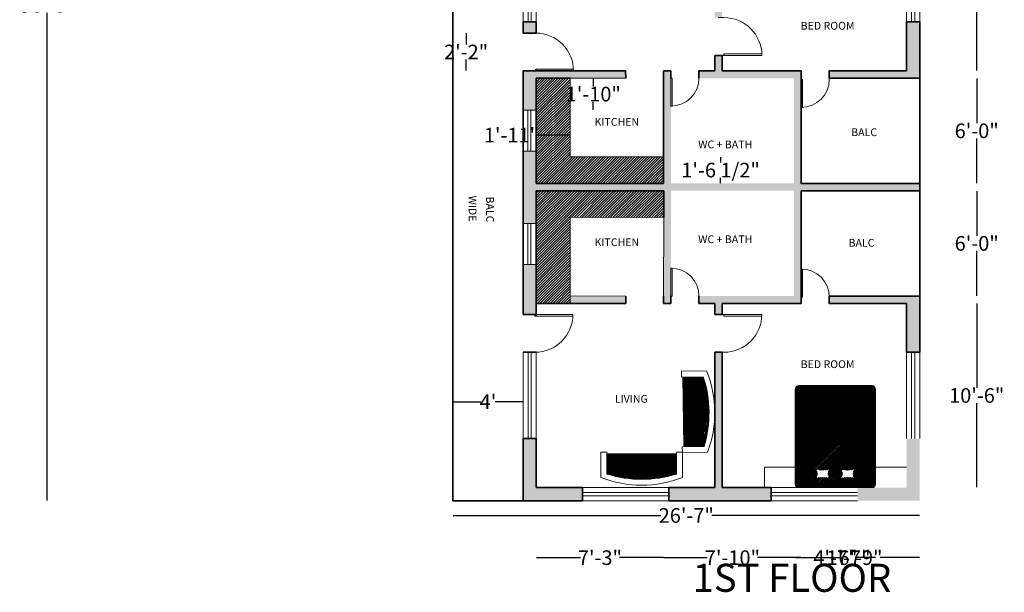
# Model space of a CAD drawing. Units: inches. Extents: x 1198 to 8596, y 144 to 930.
# Tile 1 of 5: x 1270 to 1943, y 144 to 536. Entities that reach past the tile are written whole.
import ezdxf

# ---------------------------------------------------------------- set-up
doc = ezdxf.new("R2010")
doc.units = ezdxf.units.IN
doc.header["$MEASUREMENT"] = 0
doc.layers.get('0').update_dxf_attribs({"color": 50})
for name, color, linetype, lineweight in [('A-ANNO-DIMS', 7, 'Continuous', 18), ('A-ANNO-TEXT', 7, 'Continuous', 25), ('A-AREA-IDEN', 7, 'Continuous', 18), ('A-DOOR', 120, 'Continuous', 18), ('A-FLOR-FIXT', 8, 'Continuous', 18), ('A-FLOR-FIXT-PATT', 150, 'Continuous', 13), ('A-FURN', 11, 'Continuous', 18), ('A-FURN-PATT', 11, 'Continuous', 13), ('A-WALL-PATT', 150, 'Continuous', 13), ('WALL', 7, 'Continuous', 35), ('WINDOW', 2, 'Continuous', 18)]:
    doc.layers.add(name, color=color, linetype=linetype, lineweight=lineweight)
doc.styles.get("Standard").update_dxf_attribs({"font": 'arial.ttf'})
doc.dimstyles.get("Standard").update_dxf_attribs({"dimtxt": 10, "dimasz": 0.18, "dimexe": 0.18, "dimexo": 0.0625, "dimgap": 0.09, "dimtad": 0, "dimtih": 1, "dimtoh": 1, "dimdec": 0, "dimzin": 0, "dimdsep": 46, "dimlunit": 3, "dimtxsty": 'Standard', "dimcen": 0.09, "dimse1": 1, "dimse2": 1, "dimadec": 0, "dimazin": 0, "dimtfac": 1, "dimtdec": 0, "dimtofl": 0, "dimtmove": 0, "dimatfit": 3, "dimfxl": 1, "dimtolj": 1, "dimtzin": 0, "dimarcsym": 0})

# ---------------------------------------------------------------- blocks, each defined once
blk = doc.blocks.new('*D1')
at = {"layer": 'A-ANNO-DIMS', "color": 0, "lineweight": -2, "transparency": 16777216}
for p, q in [((1566.07, 274.64), (1584.99, 274.64)), ((1613.71, 274.64), (1594.78, 274.64))]:
    blk.add_line(p, q, dxfattribs=at)
at = {"layer": 'A-ANNO-DIMS', "color": 0, "transparency": 16777216}
for points in [[(1566.07, 274.67), (1566.07, 274.61), (1565.89, 274.64)], [(1613.71, 274.67), (1613.71, 274.61), (1613.89, 274.64)]]:
    blk.add_solid(points, dxfattribs=at)
at = {"layer": 'Defpoints', "color": 0, "transparency": 16777216}
for p in [(1565.89, 284.02), (1613.89, 284.02), (1565.89, 274.64)]:
    blk.add_point(p, dxfattribs=at)
at = {"layer": 'A-ANNO-DIMS', "color": 0, "transparency": 16777216, "insert": (1589.89, 274.64), "char_height": 10, "attachment_point": 5}
blk.add_mtext("\\A1;4'", dxfattribs=at)
blk = doc.blocks.new('WD_WIN4')
for p, q in [((-0.5, 0.5), (0.5, 0.5)), ((-0.5, 0.12), (0.5, 0.12)), ((-0.5, -0.12), (0.5, -0.12)), ((-0.5, -0.5), (0.5, -0.5))]:
    blk.add_line(p, q)
blk = doc.blocks.new('*U9')
for p, q in [((0, 0), (0, -6)), ((40, 0), (40, -6))]:
    blk.add_line(p, q)
blk.add_lwpolyline([(0, 0), (0, 40), (1.75, 40), (1.75, 0)], close=True)
blk.add_arc((0, 0), 40, 0, 90)
blk = doc.blocks.new('*U11')
for p, q in [((0, 0), (0, -6)), ((40, 0), (40, -6))]:
    blk.add_line(p, q)
blk.add_lwpolyline([(0, 0), (0, 40), (1.75, 40), (1.75, 0)], close=True)
blk.add_arc((0, 0), 40, 0, 90)
blk = doc.blocks.new('*U10')
for p, q in [((0, 0), (0, -6)), ((-40, 0), (-40, -6))]:
    blk.add_line(p, q)
blk.add_lwpolyline([(0, 0), (0, 40), (-1.75, 40), (-1.75, 0)], close=True)
blk.add_arc((0, 0), 40, 90, 180)
blk = doc.blocks.new('*D17')
at = {"layer": 'A-ANNO-DIMS', "color": 0, "lineweight": -2, "transparency": 16777216}
for p, q in [((1288.75, 884.72), (1288.75, 551.09)), ((1288.75, 207.08), (1288.75, 540.7))]:
    blk.add_line(p, q, dxfattribs=at)
at = {"layer": 'A-ANNO-DIMS', "color": 0, "transparency": 16777216}
for points in [[(1288.72, 884.72), (1288.78, 884.72), (1288.75, 884.9)], [(1288.72, 207.08), (1288.78, 207.08), (1288.75, 206.9)]]:
    blk.add_solid(points, dxfattribs=at)
at = {"layer": 'Defpoints', "color": 0, "transparency": 16777216}
for p in [(1347.89, 884.9), (1288.75, 206.9), (1347.89, 206.9)]:
    blk.add_point(p, dxfattribs=at)
at = {"layer": 'A-ANNO-DIMS', "color": 0, "transparency": 16777216, "insert": (1288.75, 545.9), "char_height": 10, "attachment_point": 5}
blk.add_mtext('\\A1;56\'-6"', dxfattribs=at)
blk = doc.blocks.new('Sofa - Roundback 7 ft.')
for p, q in [((-12.00002, -32.4421), (-12.00003, -6.5971)), ((11.99997, -32.4421), (11.99998, -6.5971)), ((-36.000027, -34), (-36.000027, -11.4696)), ((-35.999844, -13.3819), (35.9998, -13.3819)), ((35.99998, -34), (35.99998, -11.4696)), ((-36.000027, -32.4421), (35.99998, -32.4421))]:
    blk.add_line(p, q)
for points in [[(-36.000027, -34), (-42.000027, -34), (-42.000027, -8)], [(41.99998, -8), (41.99998, -34), (35.99998, -34)]]:
    blk.add_lwpolyline(points)
for centre, radius, start, end in [((0, -114.25), 114.25, 68.43141, 111.5686), ((-0.00001, -127.1968), 121.1968, 72.72033, 107.2797)]:
    blk.add_arc(centre, radius, start, end)
blk = doc.blocks.new('*D19')
at = {"layer": 'A-ANNO-DIMS', "color": 0, "lineweight": -2, "transparency": 16777216}
for p, q in [((1566.07, 196.81), (1708.03, 196.81)), ((1884.71, 196.81), (1742.74, 196.81))]:
    blk.add_line(p, q, dxfattribs=at)
at = {"layer": 'A-ANNO-DIMS', "color": 0, "transparency": 16777216}
for points in [[(1566.07, 196.84), (1566.07, 196.78), (1565.89, 196.81)], [(1884.71, 196.84), (1884.71, 196.78), (1884.89, 196.81)]]:
    blk.add_solid(points, dxfattribs=at)
at = {"layer": 'Defpoints', "color": 0, "transparency": 16777216}
for p in [(1565.89, 206.9), (1884.89, 206.9), (1565.89, 196.81)]:
    blk.add_point(p, dxfattribs=at)
at = {"layer": 'A-ANNO-DIMS', "color": 0, "transparency": 16777216, "insert": (1725.39, 196.81), "char_height": 10, "attachment_point": 5}
blk.add_mtext('\\A1;26\'-7"', dxfattribs=at)
blk = doc.blocks.new('WIN-NARROW-28IN')
for p, q in [((0, 9), (0, 0)), ((28.06, 9), (28.06, 0)), ((0, 5.31), (28.06, 5.31)), ((0, 3.31), (28.06, 3.31))]:
    blk.add_line(p, q)
blk = doc.blocks.new('NIGHTSTAND')
for p, q in [((23.07, 13.96), (0, 13.96)), ((23.07, 0), (23.07, 13.96)), ((1.94, 0), (23.07, 0))]:
    blk.add_line(p, q)
blk = doc.blocks.new('*D44')
at = {"layer": 'A-ANNO-DIMS', "color": 0, "lineweight": -2, "transparency": 16777216}
for p, q in [((1923.84, 626.72), (1923.84, 569.09)), ((1923.84, 501.08), (1923.84, 558.7))]:
    blk.add_line(p, q, dxfattribs=at)
at = {"layer": 'A-ANNO-DIMS', "color": 0, "transparency": 16777216}
for points in [[(1923.81, 626.72), (1923.87, 626.72), (1923.84, 626.9)], [(1923.81, 501.08), (1923.87, 501.08), (1923.84, 500.9)]]:
    blk.add_solid(points, dxfattribs=at)
at = {"layer": 'Defpoints', "color": 0, "transparency": 16777216}
for p in [(1875.89, 626.9), (1923.84, 626.9), (1875.89, 500.9)]:
    blk.add_point(p, dxfattribs=at)
at = {"layer": 'A-ANNO-DIMS', "color": 0, "transparency": 16777216, "insert": (1923.84, 563.9), "char_height": 10, "attachment_point": 5}
blk.add_mtext('\\A1;10\'-6"', dxfattribs=at)
blk = doc.blocks.new('*D45')
at = {"layer": 'A-ANNO-DIMS', "color": 0, "lineweight": -2, "transparency": 16777216}
for p, q in [((1923.84, 495.72), (1923.84, 465.09)), ((1923.84, 424.08), (1923.84, 454.7))]:
    blk.add_line(p, q, dxfattribs=at)
at = {"layer": 'A-ANNO-DIMS', "color": 0, "transparency": 16777216}
for points in [[(1923.81, 495.72), (1923.87, 495.72), (1923.84, 495.9)], [(1923.81, 424.08), (1923.87, 424.08), (1923.84, 423.9)]]:
    blk.add_solid(points, dxfattribs=at)
at = {"layer": 'Defpoints', "color": 0, "transparency": 16777216}
for p in [(1884.89, 495.9), (1923.84, 495.9), (1884.89, 423.9)]:
    blk.add_point(p, dxfattribs=at)
at = {"layer": 'A-ANNO-DIMS', "color": 0, "transparency": 16777216, "insert": (1923.84, 459.9), "char_height": 10, "attachment_point": 5}
blk.add_mtext('\\A1;6\'-0"', dxfattribs=at)
blk = doc.blocks.new('*D46')
at = {"layer": 'A-ANNO-DIMS', "color": 0, "lineweight": -2, "transparency": 16777216}
for p, q in [((1923.84, 418.72), (1923.84, 388.09)), ((1923.84, 347.08), (1923.84, 377.7))]:
    blk.add_line(p, q, dxfattribs=at)
at = {"layer": 'A-ANNO-DIMS', "color": 0, "transparency": 16777216}
for points in [[(1923.81, 418.72), (1923.87, 418.72), (1923.84, 418.9)], [(1923.81, 347.08), (1923.87, 347.08), (1923.84, 346.9)]]:
    blk.add_solid(points, dxfattribs=at)
at = {"layer": 'Defpoints', "color": 0, "transparency": 16777216}
for p in [(1884.89, 418.9), (1923.84, 418.9), (1884.89, 346.9)]:
    blk.add_point(p, dxfattribs=at)
at = {"layer": 'A-ANNO-DIMS', "color": 0, "transparency": 16777216, "insert": (1923.84, 382.9), "char_height": 10, "attachment_point": 5}
blk.add_mtext('\\A1;6\'-0"', dxfattribs=at)
blk = doc.blocks.new('*D47')
at = {"layer": 'A-ANNO-DIMS', "color": 0, "lineweight": -2, "transparency": 16777216}
for p, q in [((1923.84, 341.72), (1923.84, 284.09)), ((1923.84, 216.08), (1923.84, 273.7))]:
    blk.add_line(p, q, dxfattribs=at)
at = {"layer": 'A-ANNO-DIMS', "color": 0, "transparency": 16777216}
for points in [[(1923.81, 341.72), (1923.87, 341.72), (1923.84, 341.9)], [(1923.81, 216.08), (1923.87, 216.08), (1923.84, 215.9)]]:
    blk.add_solid(points, dxfattribs=at)
at = {"layer": 'Defpoints', "color": 0, "transparency": 16777216}
for p in [(1875.89, 341.9), (1923.84, 341.9), (1749.89, 215.9)]:
    blk.add_point(p, dxfattribs=at)
at = {"layer": 'A-ANNO-DIMS', "color": 0, "transparency": 16777216, "insert": (1923.84, 278.9), "char_height": 10, "attachment_point": 5}
blk.add_mtext('\\A1;10\'-6"', dxfattribs=at)
blk = doc.blocks.new('*D48')
at = {"layer": 'A-ANNO-DIMS', "color": 0, "lineweight": -2, "transparency": 16777216}
for p, q in [((1623.07, 167.95), (1653.05, 167.95)), ((1709.71, 167.95), (1679.73, 167.95))]:
    blk.add_line(p, q, dxfattribs=at)
at = {"layer": 'A-ANNO-DIMS', "color": 0, "transparency": 16777216}
for points in [[(1623.07, 167.98), (1623.07, 167.92), (1622.89, 167.95)], [(1709.71, 167.98), (1709.71, 167.92), (1709.89, 167.95)]]:
    blk.add_solid(points, dxfattribs=at)
at = {"layer": 'Defpoints', "color": 0, "transparency": 16777216}
for p in [(1622.89, 341.9), (1709.89, 341.9), (1709.89, 167.95)]:
    blk.add_point(p, dxfattribs=at)
at = {"layer": 'A-ANNO-DIMS', "color": 0, "transparency": 16777216, "insert": (1666.39, 167.95), "char_height": 10, "attachment_point": 5}
blk.add_mtext('\\A1;7\'-3"', dxfattribs=at)
blk = doc.blocks.new('*D49')
at = {"layer": 'A-ANNO-DIMS', "color": 0, "lineweight": -2, "transparency": 16777216}
for p, q in [((1710.07, 167.95), (1739.68, 167.95)), ((1803.75, 167.95), (1774.13, 167.95))]:
    blk.add_line(p, q, dxfattribs=at)
at = {"layer": 'A-ANNO-DIMS', "color": 0, "transparency": 16777216}
for points in [[(1710.07, 167.98), (1710.07, 167.92), (1709.89, 167.95)], [(1803.75, 167.98), (1803.75, 167.92), (1803.93, 167.95)]]:
    blk.add_solid(points, dxfattribs=at)
at = {"layer": 'Defpoints', "color": 0, "transparency": 16777216}
for p in [(1709.89, 341.9), (1803.93, 341.9), (1803.93, 167.95)]:
    blk.add_point(p, dxfattribs=at)
at = {"layer": 'A-ANNO-DIMS', "color": 0, "transparency": 16777216, "insert": (1756.91, 167.95), "char_height": 10, "attachment_point": 5}
blk.add_mtext('\\A1;7\'-10"', dxfattribs=at)
blk = doc.blocks.new('*D50')
at = {"layer": 'A-ANNO-DIMS', "color": 0, "lineweight": -2, "transparency": 16777216}
for p, q in [((1804.07, 167.95), (1830.98, 167.95)), ((1884.71, 167.95), (1857.79, 167.95))]:
    blk.add_line(p, q, dxfattribs=at)
at = {"layer": 'A-ANNO-DIMS', "color": 0, "transparency": 16777216}
for points in [[(1804.07, 167.98), (1804.07, 167.92), (1803.89, 167.95)], [(1884.71, 167.98), (1884.71, 167.92), (1884.89, 167.95)]]:
    blk.add_solid(points, dxfattribs=at)
at = {"layer": 'Defpoints', "color": 0, "transparency": 16777216}
for p in [(1803.89, 346.9), (1884.89, 346.9), (1884.89, 167.95)]:
    blk.add_point(p, dxfattribs=at)
at = {"layer": 'A-ANNO-DIMS', "color": 0, "transparency": 16777216, "insert": (1844.39, 167.95), "char_height": 10, "attachment_point": 5}
blk.add_mtext('\\A1;6\'-9"', dxfattribs=at)
blk = doc.blocks.new('*D51')
at = {"layer": 'A-ANNO-DIMS', "color": 0, "lineweight": -2, "transparency": 16777216}
for p, q in [((1804.07, 167.95), (1822.93, 167.95)), ((1823.11, 167.95), (1823.29, 167.95))]:
    blk.add_line(p, q, dxfattribs=at)
at = {"layer": 'A-ANNO-DIMS', "color": 0, "transparency": 16777216}
for points in [[(1804.07, 167.98), (1804.07, 167.92), (1803.89, 167.95)], [(1822.93, 167.98), (1822.93, 167.92), (1823.11, 167.95)]]:
    blk.add_solid(points, dxfattribs=at)
at = {"layer": 'Defpoints', "color": 0, "transparency": 16777216}
for p in [(1803.89, 495.9), (1823.11, 495.9), (1823.11, 167.95)]:
    blk.add_point(p, dxfattribs=at)
at = {"layer": 'A-ANNO-DIMS', "color": 0, "transparency": 16777216, "insert": (1836.2, 167.95), "char_height": 10, "attachment_point": 5}
blk.add_mtext('\\A1;1\'-7"', dxfattribs=at)
blk = doc.blocks.new('*D52')
at = {"layer": 'A-ANNO-DIMS', "color": 0, "lineweight": -2, "transparency": 16777216}
for p, q in [((1574.94, 526.59), (1574.94, 518.95)), ((1574.94, 501.08), (1574.94, 508.72))]:
    blk.add_line(p, q, dxfattribs=at)
at = {"layer": 'A-ANNO-DIMS', "color": 0, "transparency": 16777216}
for points in [[(1574.91, 526.59), (1574.97, 526.59), (1574.94, 526.77)], [(1574.91, 501.08), (1574.97, 501.08), (1574.94, 500.9)]]:
    blk.add_solid(points, dxfattribs=at)
at = {"layer": 'Defpoints', "color": 0, "transparency": 16777216}
for p in [(1574.94, 526.77), (1613.89, 526.77), (1613.89, 500.9)]:
    blk.add_point(p, dxfattribs=at)
at = {"layer": 'A-ANNO-DIMS', "color": 0, "transparency": 16777216, "insert": (1574.94, 513.84), "char_height": 10, "attachment_point": 5}
blk.add_mtext('\\A1;2\'-2"', dxfattribs=at)
blk = doc.blocks.new('*D53')
at = {"layer": 'A-ANNO-DIMS', "color": 0, "lineweight": -2, "transparency": 16777216}
for p, q in [((1800.03, 167.95), (1813.72, 167.95)), ((1854.57, 167.95), (1840.88, 167.95))]:
    blk.add_line(p, q, dxfattribs=at)
at = {"layer": 'A-ANNO-DIMS', "color": 0, "transparency": 16777216}
for points in [[(1800.03, 167.98), (1800.03, 167.92), (1799.85, 167.95)], [(1854.57, 167.98), (1854.57, 167.92), (1854.75, 167.95)]]:
    blk.add_solid(points, dxfattribs=at)
at = {"layer": 'Defpoints', "color": 0, "transparency": 16777216}
for p in [(1799.85, 559.62), (1854.75, 559.62), (1854.75, 167.95)]:
    blk.add_point(p, dxfattribs=at)
at = {"layer": 'A-ANNO-DIMS', "color": 0, "transparency": 16777216, "insert": (1827.3, 167.95), "char_height": 10, "attachment_point": 5}
blk.add_mtext('\\A1;4\'-7"', dxfattribs=at)
blk = doc.blocks.new('*D62')
at = {"layer": 'A-ANNO-DIMS', "color": 0, "lineweight": -2, "transparency": 16777216}
for p, q in [((1622.89, 456.95), (1622.71, 456.95)), ((1645.75, 456.95), (1623.07, 456.95))]:
    blk.add_line(p, q, dxfattribs=at)
at = {"layer": 'A-ANNO-DIMS', "color": 0, "transparency": 16777216}
for points in [[(1623.07, 456.98), (1623.07, 456.92), (1622.89, 456.95)], [(1645.75, 456.98), (1645.75, 456.92), (1645.93, 456.95)]]:
    blk.add_solid(points, dxfattribs=at)
at = {"layer": 'Defpoints', "color": 0, "transparency": 16777216}
for p in [(1622.89, 495.9), (1645.93, 495.9), (1622.89, 456.95)]:
    blk.add_point(p, dxfattribs=at)
at = {"layer": 'A-ANNO-DIMS', "color": 0, "transparency": 16777216, "insert": (1605.91, 456.95), "char_height": 10, "attachment_point": 5}
blk.add_mtext('\\A1;1\'-11"', dxfattribs=at)
blk = doc.blocks.new('*D63')
at = {"layer": 'A-ANNO-DIMS', "color": 0, "lineweight": -2, "transparency": 16777216}
for p, q in [((1748.84, 441.97), (1748.84, 438.28)), ((1748.84, 424.08), (1748.84, 427.76))]:
    blk.add_line(p, q, dxfattribs=at)
at = {"layer": 'A-ANNO-DIMS', "color": 0, "transparency": 16777216}
for points in [[(1748.81, 441.97), (1748.87, 441.97), (1748.84, 442.15)], [(1748.81, 424.08), (1748.87, 424.08), (1748.84, 423.9)]]:
    blk.add_solid(points, dxfattribs=at)
at = {"layer": 'Defpoints', "color": 0, "transparency": 16777216}
for p in [(1709.89, 442.15), (1709.89, 423.9), (1748.84, 423.9)]:
    blk.add_point(p, dxfattribs=at)
at = {"layer": 'A-ANNO-DIMS', "color": 0, "transparency": 16777216, "insert": (1748.84, 433.02), "char_height": 10, "attachment_point": 5}
blk.add_mtext('\\A1;1\'-6 1/2"', dxfattribs=at)
blk = doc.blocks.new('*D67')
at = {"layer": 'A-ANNO-DIMS', "color": 0, "lineweight": -2, "transparency": 16777216}
for p, q in [((1661.84, 495.72), (1661.84, 490.21)), ((1661.84, 474.31), (1661.84, 479.82))]:
    blk.add_line(p, q, dxfattribs=at)
at = {"layer": 'A-ANNO-DIMS', "color": 0, "transparency": 16777216}
for points in [[(1661.81, 495.72), (1661.87, 495.72), (1661.84, 495.9)], [(1661.81, 474.31), (1661.87, 474.31), (1661.84, 474.13)]]:
    blk.add_solid(points, dxfattribs=at)
at = {"layer": 'Defpoints', "color": 0, "transparency": 16777216}
for p in [(1622.89, 495.9), (1622.89, 474.13), (1661.84, 474.13)]:
    blk.add_point(p, dxfattribs=at)
at = {"layer": 'A-ANNO-DIMS', "color": 0, "transparency": 16777216, "insert": (1661.84, 485.01), "char_height": 10, "attachment_point": 5}
blk.add_mtext('\\A1;1\'-10"', dxfattribs=at)

msp = doc.modelspace()

# ---------------------------------------------------------------- hatches: boundary and pattern name
at = {"layer": 'A-FLOR-FIXT-PATT'}
h = msp.add_hatch(dxfattribs=at)
h.set_pattern_fill('ANSI31', color=256, scale=10)
h.paths.add_polyline_path([(1646.14, 400.75), (1710.09, 400.51), (1710.09, 418.9), (1622.89, 418.9), (1622.89, 341.9), (1645.93, 341.9), (1645.93, 347.01)])
h.paths.add_polyline_path([(1709.89, 442.15), (1645.93, 442.15), (1645.93, 495.9), (1622.89, 495.9), (1622.89, 423.9), (1709.89, 423.9)])
at = {"layer": 'A-FURN-PATT'}
h = msp.add_hatch(dxfattribs=at)
h.set_pattern_fill('LINE', color=256, scale=5, angle=90.6803)
h.set_pattern_definition([(90.6803, (2441.98376, -1260.8571), (-0.62495594, -0.00742075), [])])
h.paths.add_polyline_path([(1723.51, 259.75), (1723.69, 243.86), (1736.31, 244.01), (1736.12, 259.9)])
h.paths.add_polyline_path([(1723.32, 275.63), (1723.51, 259.75), (1736.12, 259.9), (1735.93, 275.78)])
h.paths.add_polyline_path([(1723.13, 291.52), (1723.32, 275.63), (1735.93, 275.78), (1735.75, 291.67)])
h.paths.add_polyline_path([(1737.01, 291.69), (1735.75, 291.67), (1735.93, 275.78), (1740.43, 275.84, 0.050647)])
h.paths.add_polyline_path([(1735.93, 275.78), (1736.12, 259.9), (1740.61, 259.95, 0.049628), (1740.43, 275.84)])
h.paths.add_polyline_path([(1736.12, 259.9), (1736.31, 244.01), (1737.58, 244.03, 0.050647), (1740.61, 259.95)])
h = msp.add_hatch(dxfattribs=at)
h.set_pattern_fill('PLASTI', color=256, scale=6.190048)
h.set_pattern_definition([(0, (526.78, -195.5534), (0, 1.547512), []), (0, (526.78, -195.36), (0, 1.547512), []), (0, (526.78, -195.1665), (0, 1.547512), []), (0, (526.78, -194.5862), (0, 1.547512), [])])
h.paths.add_polyline_path([(1846.77, 215.84), (1852.27, 215.84, 0.414214), (1854.75, 218.31), (1854.75, 283.17, 0.414214), (1852.27, 285.65), (1846.77, 285.65)])
h.paths.add_polyline_path([(1799.85, 218.31, 0.414214), (1802.33, 215.84), (1807.83, 215.84), (1807.83, 285.65), (1802.33, 285.65, 0.414214), (1799.85, 283.17)])
h = msp.add_hatch(dxfattribs=at)
h.set_pattern_fill('ANSI38', color=256, scale=6.190048)
h.set_pattern_definition([(45, (526.78, -195.5534), (-0.5471281, 0.5471281), []), (135, (526.78, -195.5534), (-1.6413843, 0.5471281), [1.93439, -1.160634])])
h.paths.add_polyline_path([(1807.83, 215.84), (1846.77, 215.84), (1846.77, 285.65), (1807.83, 285.65)])
h.paths.add_polyline_path([(1823.26, 228.35, 0.358285), (1823.26, 222.35, 0.116256), (1813.93, 222.35, 0.358285), (1813.93, 228.35, 0.116256)], flags=16)
h.paths.add_polyline_path([(1831.01, 228.35, 0.116256), (1840.34, 228.35, 0.358285), (1840.34, 222.35, 0.116256), (1831.01, 222.35, 0.358285)], flags=16)
h = msp.add_hatch(dxfattribs=at)
h.set_pattern_fill('LINE', color=256, scale=5)
h.set_pattern_definition([(0, (157.9337, -461.3583), (0, 0.625), [])])
h.paths.add_polyline_path([(1686.96, 239.01), (1671.07, 239.01), (1671.07, 226.4), (1686.96, 226.4)])
h.paths.add_polyline_path([(1702.85, 239.01), (1686.96, 239.01), (1686.96, 226.4), (1702.85, 226.4)])
h.paths.add_polyline_path([(1718.74, 239.01), (1702.85, 239.01), (1702.85, 226.4), (1718.74, 226.4)])
h.paths.add_polyline_path([(1718.74, 225.13), (1718.74, 226.4), (1702.85, 226.4), (1702.85, 221.9, 0.050647)])
h.paths.add_polyline_path([(1702.85, 226.4), (1686.96, 226.4), (1686.96, 221.9, 0.049628), (1702.85, 221.9)])
h.paths.add_polyline_path([(1686.96, 226.4), (1671.07, 226.4), (1671.07, 225.13, 0.050647), (1686.96, 221.9)])
at = {"layer": 'A-WALL-PATT'}
h = msp.add_hatch(color=256, dxfattribs=at)
h.dxf.hatch_style = 1
h.paths.add_polyline_path([(1884.89, 495.9), (1884.89, 534.37), (1875.89, 534.37), (1875.89, 500.9), (1823.11, 500.9), (1823.11, 495.9)])
h.paths.add_polyline_path([(1875.89, 593.42), (1884.89, 593.42), (1884.89, 685.87), (1875.89, 685.87), (1875.89, 631.9), (1749.89, 631.9), (1749.89, 766.08), (1744.89, 766.08), (1744.89, 631.97), (1618.79, 631.97), (1613.89, 631.97), (1613.89, 593.42), (1622.89, 593.42), (1622.89, 626.9), (1744.89, 626.9), (1744.89, 537.33), (1749.89, 537.33), (1749.89, 626.9), (1875.89, 626.9)])
h.paths.add_polyline_path([(1884.89, 206.9), (1884.89, 249.37), (1875.89, 249.37), (1875.89, 215.9), (1842.41, 215.9), (1842.41, 206.9)])
h.paths.add_polyline_path([(1783.36, 206.9), (1783.36, 215.9), (1749.89, 215.9), (1749.89, 308.42), (1744.89, 308.42), (1744.89, 215.9), (1713.41, 215.9), (1713.41, 206.9)])
h.paths.add_polyline_path([(1654.36, 206.9), (1654.36, 215.9), (1622.89, 215.9), (1622.89, 249.37), (1613.89, 249.37), (1613.89, 206.9)])
h.paths.add_polyline_path([(1613.89, 334.34), (1622.89, 334.34), (1622.89, 341.9), (1622.89, 368.41), (1613.89, 368.41)])
h.paths.add_polyline_path([(1613.89, 396.47), (1622.89, 396.47), (1622.89, 418.9), (1710.09, 418.9), (1710.09, 400.51), (1709.89, 346.77), (1709.89, 341.9), (1714.89, 341.9), (1714.89, 346.9), (1714.88, 366), (1714.89, 418.9), (1798.89, 418.9), (1798.89, 346.9), (1734.06, 346.9), (1734.07, 343.96), (1734.06, 341.9), (1744.89, 341.9), (1744.89, 334.34), (1749.89, 334.34), (1749.89, 341.9), (1803.93, 341.9), (1803.93, 346.9), (1803.89, 346.9), (1803.89, 418.9), (1884.89, 418.9), (1884.89, 423.9), (1803.89, 423.9), (1803.89, 495.9), (1803.93, 500.9), (1749.89, 500.9), (1749.89, 511.41), (1747.24, 511.41), (1744.89, 511.41), (1744.89, 500.9), (1734.06, 500.9), (1734.06, 495.9), (1798.89, 495.9), (1798.89, 423.9), (1714.89, 423.9), (1714.89, 495.9), (1714.89, 500.9), (1709.89, 500.9), (1709.89, 496.89), (1709.89, 495.9), (1709.89, 423.9), (1622.89, 423.9), (1622.89, 446.07), (1613.89, 446.07)])
h.paths.add_polyline_path([(1613.89, 474.13), (1622.89, 474.13), (1622.89, 495.9), (1645.93, 495.9), (1683.97, 495.9), (1683.89, 500.9), (1648.32, 500.9), (1648.32, 500.88), (1622.41, 500.86), (1618.52, 500.86), (1613.89, 500.9)])
h.paths.add_polyline_path([(1613.89, 526.77), (1613.89, 534.37), (1622.89, 534.37), (1622.89, 526.77, -0.395914), (1648.3, 502.01), (1648.32, 502.01), (1648.32, 500.88), (1622.41, 500.86), (1622.41, 502), (1648.3, 502.01, 0.395914), (1622.89, 526.77)])
h.paths.add_polyline_path([(1875.89, 744.92), (1884.89, 744.92), (1884.89, 803.9), (1823.06, 803.9), (1823.06, 798.9), (1875.89, 798.9)])
h.paths.add_polyline_path([(1798.89, 803.9), (1734.06, 803.9), (1734.06, 802.45), (1734.06, 798.9), (1744.89, 798.9), (1744.89, 792), (1749.89, 792), (1749.89, 798.9), (1803.89, 798.9), (1803.89, 803.9), (1803.89, 884.9), (1774.16, 884.9), (1774.16, 875.9), (1798.89, 875.9)])
h.paths.add_polyline_path([(1746.09, 875.9), (1746.09, 884.9), (1693.91, 884.9), (1693.91, 875.9), (1709.89, 875.9), (1709.89, 803.9), (1709.89, 798.9), (1714.89, 798.9), (1714.89, 803.9), (1714.89, 875.9)])
h.paths.add_polyline_path([(1618.89, 798.9), (1683.96, 798.9), (1683.96, 803.9), (1618.89, 803.9), (1618.89, 875.9), (1634.86, 875.9), (1634.86, 884.9), (1597.91, 884.9), (1597.91, 875.9), (1613.89, 875.9), (1613.89, 803.9), (1548.75, 803.9), (1548.75, 798.9), (1613.89, 798.9), (1613.89, 657.88), (1618.8, 657.88)])
h.paths.add_polyline_path([(1522.89, 875.9), (1538.86, 875.9), (1538.86, 884.9), (1483.76, 884.9), (1483.76, 875.9), (1517.89, 875.9), (1517.89, 803.9), (1517.89, 802.46), (1517.89, 798.9), (1522.89, 798.9), (1522.89, 803.9)], flags=17)
h.paths.add_polyline_path([(1428.89, 884.9), (1428.89, 803.9), (1428.89, 798.9), (1482.89, 798.9), (1482.89, 678.9), (1356.89, 678.9), (1356.89, 709.37), (1347.89, 709.37), (1347.89, 577.9), (1508.89, 577.9), (1508.89, 586.9), (1356.89, 586.9), (1356.89, 673.9), (1565.89, 673.9), (1565.89, 678.9), (1487.89, 678.9), (1487.89, 798.9), (1498.72, 798.9), (1498.72, 803.9), (1433.89, 803.9), (1433.89, 875.9), (1455.69, 875.9), (1455.69, 884.9)])
h.paths.add_polyline_path([(1356.89, 798.9), (1409.72, 798.9), (1409.72, 803.9), (1347.89, 803.9), (1347.89, 768.42), (1356.89, 768.42)], flags=17)
h.paths.add_polyline_path([(1884.89, 346.9), (1823.09, 346.9, -0.008805), (1823.1, 346.22), (1823.11, 343.35), (1823.09, 341.9), (1875.89, 341.9), (1875.89, 308.42), (1884.89, 308.42)])
h = msp.add_hatch(color=256, dxfattribs=at)
h.dxf.hatch_style = 1
h.paths.add_polyline_path([(1683.97, 346.87), (1645.93, 347.01), (1645.93, 341.9), (1683.97, 341.9)])

# ---------------------------------------------------------------- linework, layer by layer
at = {"layer": 'A-FLOR-FIXT'}
msp.add_line((1645.93, 347.01), (1645.93, 341.9), dxfattribs=at)
for points in [[(1709.89, 495.9), (1709.89, 495.9), (1709.89, 442.15), (1645.93, 442.15), (1645.93, 495.9), (1683.97, 495.9)], [(1709.89, 346.77), (1710.09, 400.51), (1646.14, 400.75), (1645.93, 347.01), (1683.97, 346.87)]]:
    msp.add_lwpolyline(points, dxfattribs=at)
at = {"layer": 'A-FURN'}
for p, q in [((1807.83, 215.84), (1807.83, 285.65)), ((1846.77, 215.84), (1846.77, 285.65)), ((1854.75, 229.85), (1875.89, 229.85))]:
    msp.add_line(p, q, dxfattribs=at)
msp.add_lwpolyline([(1802.33, 215.84), (1852.27, 215.84, 0.414214), (1854.75, 218.31), (1854.75, 283.17, 0.414214), (1852.27, 285.65), (1802.33, 285.65, 0.414214), (1799.85, 283.17), (1799.85, 218.31, 0.414214)], format="xyb", close=True, dxfattribs=at)
at = {"layer": 'WALL'}
for p, q in [((1565.89, 577.9), (1565.89, 206.9)), ((1613.89, 534.37), (1613.89, 526.77)), ((1622.89, 534.37), (1613.89, 534.37)), ((1622.89, 526.77), (1622.89, 534.37)), ((1875.89, 500.9), (1875.89, 534.37)), ((1875.89, 534.37), (1884.89, 534.37)), ((1884.89, 308.42), (1884.89, 534.37)), ((1622.89, 526.77), (1613.89, 526.77)), ((1744.89, 500.9), (1744.89, 511.41)), ((1749.89, 511.41), (1744.89, 511.41)), ((1749.89, 500.9), (1749.89, 511.41)), ((1622.89, 500.9), (1613.89, 500.9)), ((1613.89, 500.9), (1613.89, 334.34)), ((1622.89, 500.9), (1622.89, 502)), ((1622.89, 500.9), (1683.89, 500.9)), ((1683.97, 495.9), (1683.89, 500.9)), ((1709.89, 496.89), (1709.89, 500.9)), ((1709.89, 500.9), (1714.89, 500.9)), ((1714.89, 495.97), (1714.89, 500.9)), ((1734.06, 495.9), (1734.06, 500.9)), ((1734.06, 500.9), (1744.89, 500.9)), ((1749.89, 500.9), (1803.93, 500.9)), ((1803.93, 495.9), (1803.93, 500.9)), ((1823.11, 495.9), (1823.11, 500.9)), ((1823.11, 500.9), (1875.89, 500.9)), ((1622.89, 423.9), (1622.89, 495.9)), ((1622.89, 495.9), (1645.93, 495.9)), ((1709.89, 496.89), (1709.89, 495.9)), ((1709.89, 495.9), (1709.89, 423.9)), ((1803.89, 495.9), (1803.93, 495.9)), ((1803.89, 423.9), (1803.89, 495.9)), ((1823.11, 495.9), (1884.89, 495.9)), ((1709.89, 423.9), (1622.89, 423.9)), ((1803.89, 423.9), (1884.89, 423.9)), ((1710.09, 418.9), (1622.89, 418.9)), ((1622.89, 418.9), (1622.89, 341.9)), ((1710.09, 400.51), (1710.09, 418.9)), ((1803.89, 346.9), (1803.89, 418.9)), ((1803.89, 418.9), (1884.89, 418.9)), ((1683.97, 346.9), (1683.97, 341.9)), ((1709.89, 346.9), (1709.89, 341.9)), ((1714.89, 346.9), (1714.89, 341.9)), ((1734.06, 346.9), (1734.06, 341.9)), ((1803.89, 346.9), (1804.77, 346.9)), ((1803.93, 346.9), (1803.93, 341.9)), ((1823.09, 346.9), (1823.09, 341.9)), ((1823.09, 346.9), (1884.89, 346.9)), ((1622.89, 341.9), (1683.97, 341.9)), ((1622.89, 333.21), (1622.89, 341.9)), ((1709.89, 341.9), (1714.89, 341.9)), ((1734.06, 341.9), (1744.89, 341.9)), ((1744.89, 334.34), (1744.89, 341.9)), ((1749.89, 341.9), (1803.93, 341.9)), ((1749.89, 334.34), (1749.89, 341.9)), ((1823.09, 341.9), (1875.89, 341.9)), ((1875.89, 308.42), (1875.89, 341.9)), ((1622.89, 334.34), (1613.89, 334.34)), ((1749.89, 334.34), (1744.89, 334.34)), ((1622.89, 308.42), (1613.89, 308.42)), ((1622.89, 308.42), (1622.89, 308.44)), ((1744.89, 215.9), (1744.89, 308.42)), ((1749.89, 308.42), (1744.89, 308.42)), ((1749.89, 215.9), (1749.89, 308.42)), ((1875.89, 308.42), (1884.89, 308.42)), ((1613.89, 249.37), (1613.89, 206.9)), ((1622.89, 249.37), (1613.89, 249.37)), ((1622.89, 215.9), (1622.89, 249.37)), ((1622.89, 215.9), (1654.36, 215.9)), ((1654.36, 215.9), (1654.36, 206.9)), ((1713.41, 215.9), (1744.89, 215.9)), ((1713.41, 215.9), (1713.41, 206.9)), ((1749.89, 215.9), (1783.36, 215.9)), ((1783.36, 215.9), (1783.36, 206.9)), ((1565.89, 206.9), (1654.36, 206.9)), ((1713.41, 206.9), (1783.36, 206.9))]:
    msp.add_line(p, q, dxfattribs=at)

# ---------------------------------------------------------------- block references
at = {"layer": 'A-DOOR'}
for name, p, xscale, yscale, zscale, rotation in [('*U10', (1751.13, 511.41), 0.6478828703427376, 0.6478828703427376, 0.6478828703427376, 270.0341043339827), ('*U10', (1622.41, 500.86), 0.6478828703427376, 0.6478828703427376, 0.6478828703427376, 270.0341043339827), ('*U11', (1714.89, 495.97), -0.4792807635590344, 0.4792807635590344, 0.4792807635590344, 179.9658956660211), ('*U11', (1803.93, 495.09), -0.4792807635590344, 0.4792807635590344, 0.4792807635590344, 179.9658956660211), ('*U11', (1714.89, 346.82), 0.4792807635590344, 0.4792807635590344, 0.4792807635590344, 0.0341043339915428), ('*U11', (1803.93, 346.21), 0.4792807635590344, 0.4792807635590344, 0.4792807635590344, 0.0341043339915428), ('*U9', (1621.98, 334.34), 0.6478828703427376, 0.6478828703427376, 0.6478828703427376, 270), ('*U9', (1751.09, 334.34), 0.6478828703427376, 0.6478828703427376, 0.6478828703427376, 270)]:
    msp.add_blockref(name, p, dxfattribs=dict(at, xscale=xscale, yscale=yscale, zscale=zscale, rotation=rotation))
at = {"layer": 'A-FURN', "xscale": 0.6619781710857556, "yscale": 0.6619781710857556, "zscale": 0.6619781710857556}
for p, rotation in [((1744.89, 267.95), 270.6803002411188), ((1694.91, 217.54), 179.9999999999996)]:
    msp.add_blockref('Sofa - Roundback 7 ft.', p, dxfattribs=dict(at, rotation=rotation))
at = {"layer": 'A-FURN', "rotation": 180}
msp.add_blockref('NIGHTSTAND', (1801.79, 229.85), dxfattribs=at)
at = {"layer": 'WINDOW', "xscale": 59.05511811023622, "zscale": 59.05511811023622}
for p, yscale, rotation in [((1618.39, 563.9), 8.999999999999773, 90.00000000000351), ((1880.39, 563.9), 8.999999999988859, 270.0000000000092), ((1618.39, 278.9), 8.999999999982945, 90.00000000000043), ((1880.39, 278.9), 8.999999999998863, 270.0000000000002), ((1683.89, 211.4), 8.999999999972289, 9.0446e-12), ((1812.89, 211.4), 9.000000000001336, 180.0000000000002)]:
    msp.add_blockref('WD_WIN4', p, dxfattribs=dict(at, yscale=yscale, rotation=rotation))
at = {"layer": 'WINDOW', "rotation": 270.0000000000001}
for p in [(1613.89, 474.13), (1613.89, 396.47)]:
    msp.add_blockref('WIN-NARROW-28IN', p, dxfattribs=at)

# ---------------------------------------------------------------- texts
at = {"layer": 'A-ANNO-TEXT'}
msp.add_text('1ST FLOOR', height=19.187, dxfattribs=at).set_placement((1729.68, 144.57))
at = {"layer": 'A-AREA-IDEN'}
for s, p in [(' BED ROOM', (1801.94, 529.13)), (' KITCHEN', (1661.06, 463.35)), ('BALC', (1838.07, 456.29)), ('WC + BATH', (1733.51, 447.94)), (' KITCHEN', (1661.06, 381.02)), ('WC + BATH', (1733.51, 383.09)), ('BALC', (1836.29, 380.66)), (' BED ROOM', (1801.94, 297.64)), (' LIVING', (1674.94, 273.88))]:
    msp.add_text(s, height=5.299, dxfattribs=at).set_placement(p)
for s, p in [(' WIDE', (1576.71, 417.23)), ('BALC', (1588.61, 414.93))]:
    msp.add_text(s, height=5.299, rotation=270, dxfattribs=at).set_placement(p)

# ---------------------------------------------------------------- dimensions: what is measured, and where the dimension line sits
at = {"layer": 'A-ANNO-DIMS'}
for base, p1, p2, angle, override, picture, middle in [((1288.75, 206.9), (1347.89, 884.9), (1347.89, 206.9), 90, {"dimclrd": 0, "dimclre": 0, "dimclrt": 0}, '*D17', (1288.75, 545.9)), ((1923.84, 626.9), (1875.89, 500.9), (1875.89, 626.9), 90, {"dimdec": 1, "dimlfac": 1, "dimrnd": 0, "dimzin": 1, "dimdsep": 46, "dimlunit": 4, "dimfrac": 2}, '*D44', (1923.84, 563.9)), ((1574.94, 526.77), (1613.89, 500.9), (1613.89, 526.77), 90, {"dimdec": 1, "dimlfac": 1, "dimrnd": 0, "dimzin": 1, "dimdsep": 46, "dimlunit": 4, "dimfrac": 2}, '*D52', (1574.94, 513.84)), ((1622.89, 456.95), (1645.93, 495.9), (1622.89, 495.9), 180, {"dimdec": 1, "dimlfac": 1, "dimrnd": 0, "dimzin": 1, "dimdsep": 46, "dimlunit": 4, "dimfrac": 2}, '*D62', (1605.91, 456.95)), ((1661.84, 474.13), (1622.89, 495.9), (1622.89, 474.13), 270, {"dimdec": 1, "dimlfac": 1, "dimrnd": 0, "dimzin": 1, "dimdsep": 46, "dimlunit": 4, "dimfrac": 2}, '*D67', (1661.84, 485.01)), ((1923.84, 495.9), (1884.89, 423.9), (1884.89, 495.9), 90, {"dimdec": 1, "dimlfac": 1, "dimrnd": 0, "dimzin": 1, "dimdsep": 46, "dimlunit": 4, "dimfrac": 2}, '*D45', (1923.84, 459.9)), ((1748.8363, 423.8966), (1709.8863, 442.1522), (1709.8863, 423.8966), 270, {"dimdec": 1, "dimlfac": 1, "dimrnd": 0, "dimzin": 1, "dimdsep": 46, "dimlunit": 4, "dimfrac": 2}, '*D63', (1748.8363, 433.0244)), ((1923.84, 418.9), (1884.89, 346.9), (1884.89, 418.9), 90, {"dimdec": 1, "dimlfac": 1, "dimrnd": 0, "dimzin": 1, "dimdsep": 46, "dimlunit": 4, "dimfrac": 2}, '*D46', (1923.84, 382.9)), ((1923.84, 341.9), (1749.89, 215.9), (1875.89, 341.9), 90, {"dimdec": 1, "dimlfac": 1, "dimrnd": 0, "dimzin": 1, "dimdsep": 46, "dimlunit": 4, "dimfrac": 2}, '*D47', (1923.84, 278.9))]:
    dim = msp.add_linear_dim(base=base, p1=p1, p2=p2, angle=angle, dimstyle='Standard', override=override, dxfattribs=at)
    dim.commit()
    dim.dimension.update_dxf_attribs({"geometry": picture, "text_midpoint": middle})
for base, p1, p2, override, picture, middle in [((1854.75, 167.95), (1799.85, 559.62), (1854.75, 559.62), {"dimdec": 1, "dimlfac": 1, "dimrnd": 0, "dimzin": 1, "dimdsep": 46, "dimlunit": 4, "dimfrac": 2}, '*D53', (1827.3, 167.95)), ((1823.11, 167.95), (1803.89, 495.9), (1823.11, 495.9), {"dimdec": 1, "dimlfac": 1, "dimrnd": 0, "dimzin": 1, "dimdsep": 46, "dimlunit": 4, "dimfrac": 2}, '*D51', (1836.2, 167.95)), ((1884.89, 167.95), (1803.89, 346.9), (1884.89, 346.9), {"dimdec": 1, "dimlfac": 1, "dimrnd": 0, "dimzin": 1, "dimdsep": 46, "dimlunit": 4, "dimfrac": 2}, '*D50', (1844.39, 167.95)), ((1709.89, 167.95), (1622.89, 341.9), (1709.89, 341.9), {"dimdec": 1, "dimlfac": 1, "dimrnd": 0, "dimzin": 1, "dimdsep": 46, "dimlunit": 4, "dimfrac": 2}, '*D48', (1666.39, 167.95)), ((1803.93, 167.95), (1709.89, 341.9), (1803.93, 341.9), {"dimdec": 1, "dimlfac": 1, "dimrnd": 0, "dimzin": 1, "dimdsep": 46, "dimlunit": 4, "dimfrac": 2}, '*D49', (1756.91, 167.95)), ((1565.89, 274.64), (1613.89, 284.02), (1565.89, 284.02), {"dimclrd": 0, "dimclre": 0, "dimclrt": 0}, '*D1', (1589.89, 274.64)), ((1565.89, 196.81), (1884.89, 206.9), (1565.89, 206.9), {"dimclrd": 0, "dimclre": 0, "dimclrt": 0}, '*D19', (1725.39, 196.81))]:
    dim = msp.add_linear_dim(base=base, p1=p1, p2=p2, dimstyle='Standard', override=override, dxfattribs=at)
    dim.commit()
    dim.dimension.update_dxf_attribs({"geometry": picture, "text_midpoint": middle})

doc.saveas('drawing.dxf')
